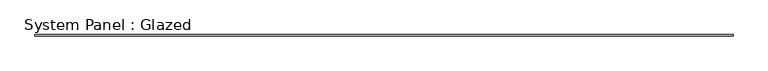
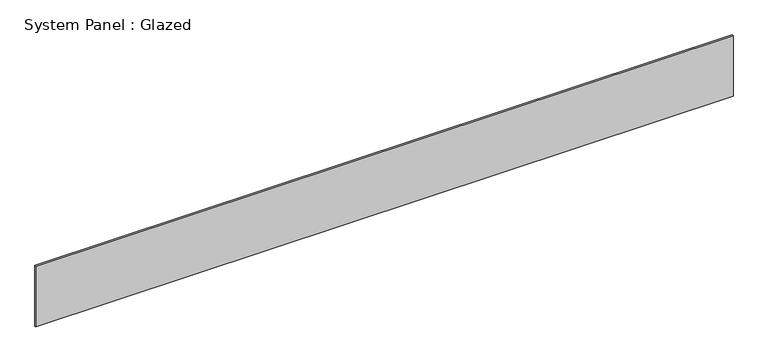
"""IFC4 building model written with IfcOpenShell, lengths in millimetres: plate geometry, System Panel : Glazed."""

from ifc_helpers import new_model, si_unit, origin, origin_with_axes, place, context, project, spatial, polyline, outline, extrude, source, transform, mapped, element, save


def system_panel_glazed_689d74eb(model_context):
    return source(origin(), model_context, "Body", "SweptSolid", [
        extrude(outline(polyline([(6277.7776373, 19.05), (-6277.7776373, 19.05), (-6277.7776373, 44.45), (6277.7776373, 44.45), (6277.7776373, 19.05)])), origin_with_axes(), (0.0, 0.0, 1.0), 1155.7),
    ])


if __name__ == "__main__":
    model = new_model("IFC4")
    model_context = context("Model", 3, world=origin())
    ifc_project = project(units=[si_unit("LENGTHUNIT", "METRE", prefix="MILLI")], contexts=[model_context])
    site = spatial("IfcSite", under=ifc_project)
    building = spatial("IfcBuilding", under=site)
    placement = place(None, origin())
    system_panel_glazed_shape = system_panel_glazed_689d74eb(model_context)
    element("IfcPlate", 1, ObjectType="System Panel : Glazed", at=placement, inside=building, context=model_context, shape_type="MappedRepresentation", body=[
        mapped(system_panel_glazed_shape, transform((0.0, 0.0, 0.0), x_axis=(1.0, 0.0, 0.0), y_axis=(0.0, 1.0, 0.0), z_axis=(0.0, 0.0, 1.0))),
    ])
    save(model, "model.ifc")

# Revit data of these elements
# Type "System Panel : Glazed"
#   Construction Type Id = "GSP4R"
#   Analytic Construction = "1/8 in Pilkington single glazing"
#   Visual Light Transmittance = 0.9
#   Solar Heat Gain Coefficient = 0.86
#   Heat Transfer Coefficient (U) = 1.18115 BTU/(h·ft²·°F)
# Element 1 (IfcPlate, "System Panel : Glazed")
#   Materials on its faces: "Glass"
# Materials
#   "Glass": class "Glass", colour RGB 0 128 192, transparency 0.75, Description = "Soda Lime Glass", Cost = 0
